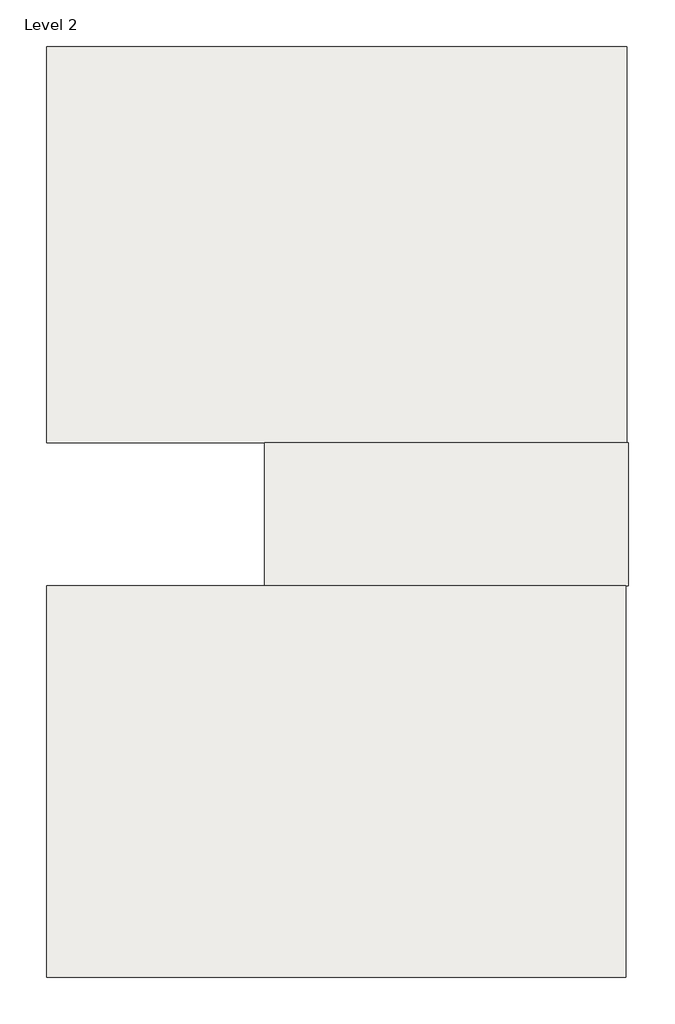
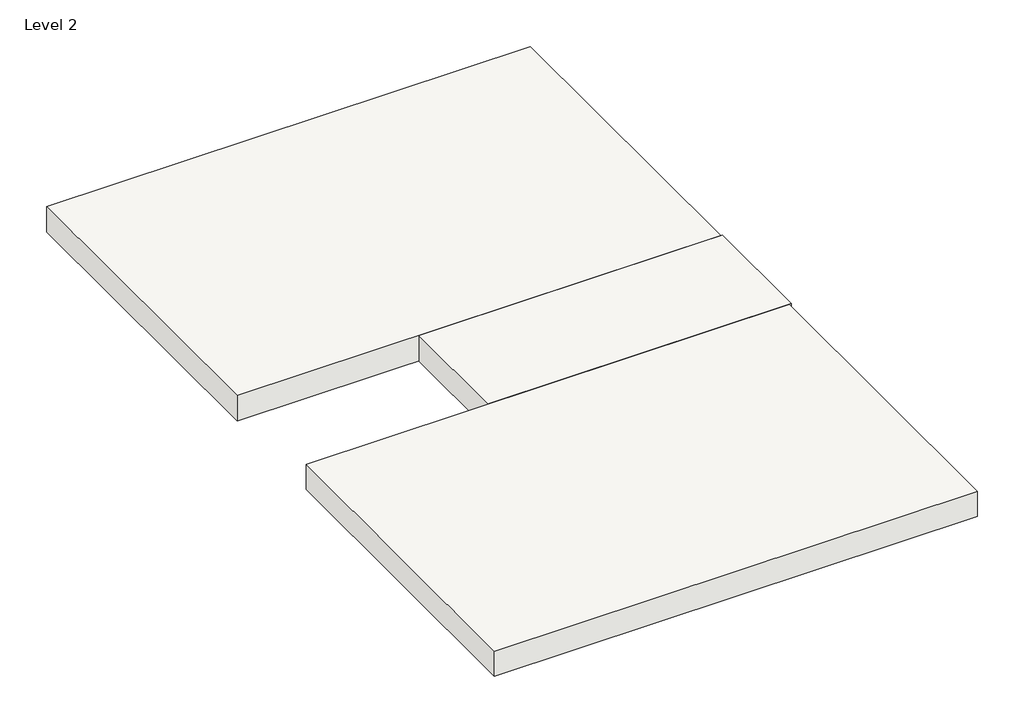
# One storey: 3 roofs.
"""IFC4 building model written with IfcOpenShell, lengths in millimetres."""

from ifc_helpers import new_model, si_unit, frame, origin, place, context, project, spatial, polyline, outline, extrude, element, save

model = new_model("IFC4")

# Units and contexts
model_context = context("Model", 3, world=origin())
ifc_project = project(units=[si_unit("LENGTHUNIT", "METRE", prefix="MILLI")], contexts=[model_context])

# Site, building, storey
site = spatial("IfcSite", under=ifc_project)
building = spatial("IfcBuilding", under=site)
storey = spatial("IfcBuildingStorey", under=building, Name="Level 2", Elevation=3048.0)

# Roofs
placement = place(None, origin())
element("IfcRoof", 1, ObjectType="Steel Truss - Insulation on Metal Deck - EPDM", at=placement, inside=storey, context=model_context, shape_type="SweptSolid", body=[
    extrude(outline(polyline([(-14570.2750862, 5999.0620171), (-4715.0750862, 5999.0620171), (-4715.0750862, -655.7379829), (-14570.2750862, -655.7379829), (-14570.2750862, 5999.0620171)])), frame((0.0, 0.0, 3048.0), z_axis=(0.0, 0.0, 1.0), x_axis=(1.0, 0.0, 0.0)), (0.0, 0.0, 1.0), 546.1),
])
element("IfcRoof", 2, ObjectType="Steel Truss - Insulation on Metal Deck - EPDM", at=placement, inside=storey, context=model_context, shape_type="SweptSolid", body=[
    extrude(outline(polyline([(-4702.3750862, 8437.4620171), (-14570.2750862, 8437.4620171), (-14570.2750862, 15168.4620171), (-4702.3750862, 15168.4620171), (-4702.3750862, 8437.4620171)])), frame((0.0, 0.0, 3048.0), z_axis=(0.0, 0.0, 1.0), x_axis=(1.0, 0.0, 0.0)), (0.0, 0.0, 1.0), 546.1),
])
element("IfcRoof", 3, ObjectType="Steel Truss - Insulation on Metal Deck - EPDM", at=placement, inside=storey, context=model_context, shape_type="SweptSolid", body=[
    extrude(outline(polyline([(-10861.8750862, 5999.0620171), (-10861.8750862, 8437.4620171), (-4676.39479, 8437.4620171), (-4676.39479, 5999.0620171), (-10861.8750862, 5999.0620171)])), frame((0.0, 0.0, 3048.0), z_axis=(0.0, 0.0, 1.0), x_axis=(1.0, 0.0, 0.0)), (0.0, 0.0, 1.0), 546.1),
])

save(model, "model.ifc")

# Revit data of these elements
# Type "Steel Truss - Insulation on Metal Deck - EPDM"
#   Assembly Code = "B1020"
#   Layers, outside or top first: 0' - 0 1/4" "Roofing, EPDM Membrane" (function 4); 0' - 5" "Rigid insulation" (function 3); 0' - 0 1/4" "Metal Deck" (function 1); 1' - 4" "Structure, Steel Bar Joist Layer" (function 1)
# Elements 1, 2, 3 (IfcRoof, "Steel Truss - Insulation on Metal Deck - EPDM")
#   built-in parameter 1001705 = 11.7917 (stored number, unit not read)
#   built-in parameter 1001710 = 33615
#   Phase Created = New Construction
#   Materials on its faces: "Structure, Steel Bar Joist Layer", "Roofing, EPDM Membrane"
# Materials
#   "Roofing, EPDM Membrane": class "Generic", colour RGB 127 127 127, transparency 0, Description = "EPDM roof membrane", Cost = 0
#   "Rigid insulation": class "Generic", colour RGB 127 127 127, transparency 0, Description = "Rigid foam insulation board", Cost = 0
#   "Metal Deck": class "Metal", colour RGB 199 199 199, transparency 0, Description = "Steel, mill finish", Cost = 0
#   "Structure, Steel Bar Joist Layer": class "Metal", colour RGB 127 127 127, transparency 0, Description = "Bar joists, thermal airspace", Cost = 0
